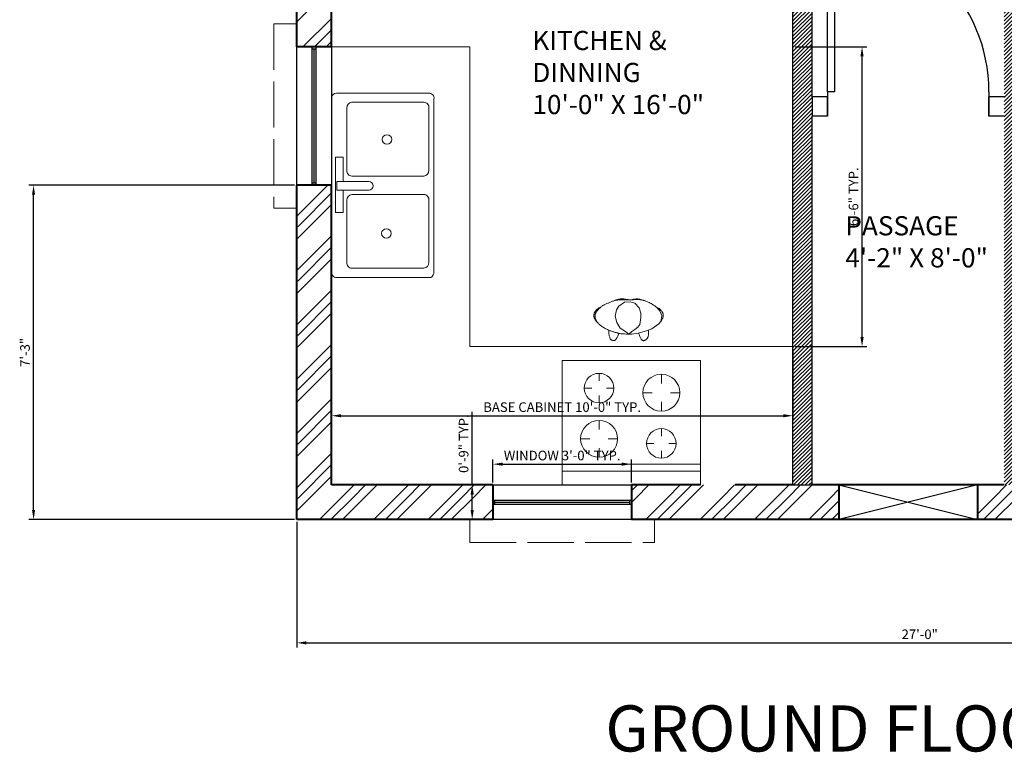
# Model space of a CAD drawing. Units: inches. Extents: x 2443635 to 2446153, y 1826255 to 1827341.
# Tile 1 of 16: x 2443635 to 2443891, y 1826801 to 1826991. Entities that reach past the tile are written whole.
import ezdxf

# ---------------------------------------------------------------- set-up
doc = ezdxf.new("R2010")
doc.units = ezdxf.units.IN
doc.linetypes.add('ACAD_ISO02W100', pattern=[15, 12, -3])
for name, color, linetype, lineweight in [('A-DIMS', 1, 'Continuous', 18), ('A-DOOR', 2, 'Continuous', 25), ('A-ENTG', 111, 'Continuous', 13), ('A-EQPM', 8, 'Continuous', 18), ('A-FLOR-CASE', 8, 'Continuous', 18), ('A-FLOR-FIXT', 9, 'Continuous', 18), ('A-ROOM', 4, 'Continuous', 18), ('A-TEXT', 4, 'Continuous', 25), ('A-WALL-EXT', 7, 'Continuous', 40), ('A-WALL-INT', 9, 'Continuous', 30), ('A-WALL-OVHD', 7, 'ACAD_ISO02W100', 18), ('A-WALL-PATT', 8, 'Continuous', 13), ('A-WINDOW', 4, 'Continuous', 25)]:
    doc.layers.add(name, color=color, linetype=linetype, lineweight=lineweight)
doc.styles.add('ATT', font='romans.shx')
doc.styles.get("Standard").update_dxf_attribs({"font": 'arial.ttf'})
doc.dimstyles.new('ISO-25', dxfattribs={"dimtxt": 2.5, "dimasz": 2.5, "dimexe": 1.25, "dimexo": 0.625, "dimtad": 1, "dimlunit": 4, "dimtxsty": 'Standard', "dimcen": 2.5, "dimadec": 0, "dimazin": 0, "dimtfac": 1, "dimtmove": 0, "dimatfit": 3, "dimfxl": 1, "dimarcsym": 0})

# ---------------------------------------------------------------- blocks, each defined once
blk = doc.blocks.new('*U2')
for p, q in [((0, 0), (0, -6)), ((40, 0), (40, -6))]:
    blk.add_line(p, q)
blk.add_lwpolyline([(0, 0), (0, 40), (1.75, 40), (1.75, 0)], close=True)
blk.add_arc((0, 0), 40, 0, 90)
blk = doc.blocks.new('11PRNG01')
at = {"color": 0, "linetype": 'ByBlock'}
for p, q in [((0, 30), (27, 30)), ((0, 0), (0, 30)), ((3, 0), (3, 30)), ((4.5, 0), (4.5, 30)), ((27, 30), (27, 0)), ((10, 26), (10, 24)), ((21, 25.2), (21, 23.6)), ((6, 22), (8, 22)), ((14, 22), (12, 22)), ((17.8, 22), (19.4, 22)), ((24.2, 22), (22.6, 22)), ((10, 18), (10, 20)), ((21, 18.8), (21, 20.4)), ((9, 11.7), (9, 10.1)), ((20, 12.5), (20, 10.5)), ((5.8, 8.5), (7.4, 8.5)), ((9, 5.3), (9, 6.9)), ((12.2, 8.5), (10.6, 8.5)), ((16, 8.5), (18, 8.5)), ((20, 4.5), (20, 6.5)), ((24, 8.5), (22, 8.5)), ((27, 0), (0, 0))]:
    blk.add_line(p, q, dxfattribs=at)
for centre, radius in [((10, 22), 4), ((21, 22), 3.2), ((9, 8.5), 3.2), ((20, 8.5), 4)]:
    blk.add_circle(centre, radius, dxfattribs=at)
at = {"color": 0, "linetype": 'ByBlock', "style": 'ATT'}
for tag, p, flags in [('ITEM', (0, -11), 3), ('ROOM_NUMBER', (0, -20), 1), ('DEPTH', (0, -29), 3), ('WIDTH', (0, -38), 3)]:
    blk.add_attdef(tag, p, '', height=6, dxfattribs=dict(at, flags=flags))
blk = doc.blocks.new('PERSON-STANDING-PLAN')
at = {"transparency": 33554687}
for p, q in [((4.62, 10.18), (4.79, 10.25)), ((4.79, 10.25), (4.96, 10.31)), ((4.96, 10.31), (5.14, 10.38)), ((5.14, 10.38), (5.33, 10.43)), ((5.33, 10.43), (5.53, 10.48)), ((5.48, 10.5), (5.36, 10.44)), ((5.69, 10.59), (5.48, 10.5)), ((5.53, 10.48), (5.74, 10.51)), ((5.91, 10.67), (5.69, 10.59)), ((5.74, 10.51), (5.95, 10.55)), ((6.13, 10.74), (5.91, 10.67)), ((5.95, 10.55), (6.17, 10.57)), ((6.35, 10.79), (6.13, 10.74)), ((6.17, 10.57), (6.39, 10.59)), ((6.57, 10.84), (6.35, 10.79)), ((6.39, 10.59), (6.61, 10.61)), ((6.79, 10.87), (6.57, 10.84)), ((6.61, 10.61), (6.83, 10.62)), ((6.99, 10.89), (6.79, 10.87)), ((6.83, 10.62), (7.05, 10.63)), ((7.18, 10.9), (6.99, 10.89)), ((7.05, 10.63), (7.26, 10.64)), ((7.38, 10.9), (7.18, 10.9)), ((7.26, 10.64), (7.47, 10.65)), ((7.57, 10.88), (7.38, 10.9)), ((7.47, 10.65), (7.68, 10.65)), ((7.78, 10.87), (7.57, 10.88)), ((7.68, 10.65), (7.87, 10.65)), ((7.99, 10.84), (7.78, 10.87)), ((7.87, 10.65), (8.06, 10.65)), ((8.22, 10.82), (7.99, 10.84)), ((8.06, 10.65), (8.23, 10.65)), ((9.71, 10.64), (8.22, 10.82)), ((8.23, 10.65), (8.39, 10.65)), ((8.39, 10.65), (8.54, 10.64)), ((8.54, 10.64), (8.67, 10.64)), ((8.67, 10.64), (8.78, 10.63)), ((8.78, 10.63), (8.89, 10.62)), ((8.89, 10.62), (8.98, 10.61)), ((8.98, 10.61), (9.08, 10.6)), ((9.08, 10.6), (9.16, 10.59)), ((9.16, 10.59), (9.25, 10.59)), ((9.25, 10.59), (9.35, 10.59)), ((9.35, 10.59), (9.44, 10.59)), ((9.44, 10.59), (9.55, 10.6)), ((9.55, 10.6), (9.66, 10.61)), ((9.9, 10.69), (9.56, 10.61)), ((9.66, 10.61), (9.78, 10.62)), ((9.78, 10.62), (9.9, 10.63)), ((10.22, 10.76), (9.9, 10.69)), ((9.9, 10.63), (10.03, 10.64)), ((10.03, 10.64), (10.16, 10.66)), ((10.16, 10.66), (10.3, 10.67)), ((10.5, 10.81), (10.22, 10.76)), ((10.3, 10.67), (10.45, 10.68)), ((10.45, 10.68), (10.61, 10.7)), ((10.76, 10.84), (10.5, 10.81)), ((10.61, 10.7), (10.76, 10.71)), ((10.99, 10.86), (10.76, 10.84)), ((10.76, 10.71), (10.92, 10.71)), ((10.92, 10.71), (11.09, 10.72)), ((11.2, 10.87), (10.99, 10.86)), ((11.09, 10.72), (11.25, 10.72)), ((11.4, 10.86), (11.2, 10.87)), ((11.25, 10.72), (11.41, 10.72)), ((11.58, 10.84), (11.4, 10.86)), ((11.41, 10.72), (11.57, 10.71)), ((11.57, 10.71), (11.73, 10.7)), ((11.76, 10.81), (11.58, 10.84)), ((11.73, 10.7), (11.89, 10.68)), ((11.93, 10.77), (11.76, 10.81)), ((11.89, 10.68), (12.04, 10.67)), ((12.11, 10.73), (11.93, 10.77)), ((12.04, 10.67), (12.19, 10.64)), ((12.29, 10.67), (12.11, 10.73)), ((12.19, 10.64), (12.34, 10.62)), ((12.48, 10.61), (12.29, 10.67)), ((12.34, 10.62), (12.48, 10.59)), ((12.68, 10.55), (12.48, 10.61)), ((12.48, 10.59), (12.62, 10.56)), ((12.62, 10.56), (12.77, 10.53)), ((12.91, 10.49), (12.68, 10.55)), ((12.77, 10.53), (12.91, 10.49)), ((12.91, 10.49), (13.05, 10.45)), ((13.17, 10.43), (12.91, 10.49)), ((13.05, 10.45), (13.2, 10.41)), ((13.2, 10.41), (13.35, 10.36)), ((13.35, 10.36), (13.51, 10.3)), ((13.51, 10.3), (13.69, 10.22)), ((0.39, 7.71), (0.32, 7.61)), ((0.48, 7.82), (0.39, 7.71)), ((0.57, 7.92), (0.48, 7.82)), ((0.67, 8.02), (0.57, 7.92)), ((0.77, 8.12), (0.67, 8.02)), ((0.76, 7.64), (0.85, 7.75)), ((0.87, 8.21), (0.77, 8.12)), ((0.85, 7.75), (0.94, 7.85)), ((0.97, 8.29), (0.87, 8.21)), ((0.94, 7.85), (1.03, 7.96)), ((1.08, 8.36), (0.97, 8.29)), ((1.03, 7.96), (1.12, 8.07)), ((1.17, 8.42), (1.08, 8.36)), ((1.12, 8.07), (1.21, 8.17)), ((1.26, 8.47), (1.17, 8.42)), ((1.21, 8.17), (1.3, 8.27)), ((1.35, 8.51), (1.26, 8.47)), ((1.3, 8.27), (1.39, 8.37)), ((1.43, 8.54), (1.35, 8.51)), ((1.39, 8.37), (1.49, 8.47)), ((1.49, 8.56), (1.43, 8.54)), ((1.55, 8.58), (1.49, 8.56)), ((1.49, 8.47), (1.59, 8.57)), ((1.59, 8.59), (1.55, 8.58)), ((1.59, 8.57), (1.69, 8.66)), ((1.62, 8.6), (1.59, 8.59)), ((1.69, 8.66), (1.79, 8.76)), ((1.79, 8.76), (1.9, 8.85)), ((1.9, 8.85), (2.01, 8.94)), ((2.01, 8.94), (2.13, 9.02)), ((2.13, 9.02), (2.26, 9.11)), ((2.26, 9.11), (2.39, 9.19)), ((2.39, 9.19), (2.54, 9.27)), ((2.54, 9.27), (2.7, 9.35)), ((2.7, 9.35), (2.86, 9.42)), ((2.86, 9.42), (3.04, 9.5)), ((3.04, 9.5), (3.21, 9.57)), ((3.21, 9.57), (3.39, 9.65)), ((3.39, 9.65), (3.58, 9.72)), ((3.58, 9.72), (3.76, 9.79)), ((3.76, 9.79), (3.94, 9.87)), ((3.94, 9.87), (4.11, 9.95)), ((4.11, 9.95), (4.28, 10.02)), ((4.28, 10.02), (4.45, 10.1)), ((4.45, 10.1), (4.62, 10.18)), ((5.88, 8.02), (5.48, 6.38)), ((6.48, 9.01), (5.88, 8.02)), ((7.91, 9.98), (6.48, 9.01)), ((9.39, 10.13), (7.91, 9.98)), ((10.63, 9.72), (9.39, 10.13)), ((11.79, 8.58), (10.63, 9.72)), ((12.18, 7.14), (11.79, 8.58)), ((13.69, 10.22), (13.89, 10.14)), ((13.89, 10.14), (14.11, 10.04)), ((14.11, 10.04), (14.35, 9.93)), ((14.35, 9.93), (14.61, 9.79)), ((14.61, 9.79), (14.89, 9.64)), ((14.89, 9.64), (15.18, 9.47)), ((15.18, 9.47), (15.49, 9.28)), ((15.49, 9.28), (15.8, 9.07)), ((15.8, 9.07), (16.12, 8.84)), ((16.12, 8.84), (16.44, 8.59)), ((16.26, 8.74), (17.17, 7.78)), ((16.44, 8.59), (16.61, 8.53)), ((16.61, 8.53), (16.77, 8.45)), ((16.77, 8.45), (16.94, 8.35)), ((16.94, 8.35), (17.1, 8.23)), ((17.1, 8.23), (17.24, 8.1)), ((17.17, 7.78), (17.68, 6.58)), ((17.24, 8.1), (17.38, 7.96)), ((17.38, 7.96), (17.51, 7.82)), ((17.51, 7.82), (17.61, 7.69)), ((17.61, 7.69), (17.7, 7.56)), ((0.01, 6.79), (0, 6.71)), ((0, 6.71), (0, 6.61)), ((0, 6.61), (0, 6.52)), ((0, 6.52), (0, 6.42)), ((0, 6.42), (0.01, 6.33)), ((0.02, 6.88), (0.01, 6.79)), ((0.01, 6.33), (0.02, 6.22)), ((0.04, 6.97), (0.02, 6.88)), ((0.02, 6.22), (0.04, 6.12)), ((0.06, 7.06), (0.04, 6.97)), ((0.04, 6.12), (0.06, 6)), ((0.08, 7.15), (0.06, 7.06)), ((0.06, 6), (0.1, 5.88)), ((0.11, 7.23), (0.08, 7.15)), ((0.1, 5.88), (0.15, 5.75)), ((0.15, 7.33), (0.11, 7.23)), ((0.2, 7.42), (0.15, 7.33)), ((0.15, 5.75), (0.23, 5.6)), ((0.25, 7.51), (0.2, 7.42)), ((0.23, 5.6), (0.33, 5.43)), ((0.32, 7.61), (0.25, 7.51)), ((0.28, 6.52), (0.29, 6.66)), ((0.29, 6.38), (0.28, 6.52)), ((0.29, 6.66), (0.31, 6.8)), ((0.3, 6.24), (0.29, 6.38)), ((0.32, 6.09), (0.3, 6.24)), ((0.31, 6.8), (0.35, 6.93)), ((0.35, 5.95), (0.32, 6.09)), ((0.33, 5.43), (0.48, 5.23)), ((0.35, 6.93), (0.4, 7.06)), ((0.39, 5.81), (0.35, 5.95)), ((0.43, 5.68), (0.39, 5.81)), ((0.4, 7.06), (0.46, 7.18)), ((0.48, 5.55), (0.43, 5.68)), ((0.46, 7.18), (0.52, 7.3)), ((0.53, 5.42), (0.48, 5.55)), ((0.48, 5.23), (0.67, 5.01)), ((0.52, 7.3), (0.6, 7.41)), ((0.58, 5.3), (0.53, 5.42)), ((0.64, 5.19), (0.58, 5.3)), ((0.6, 7.41), (0.68, 7.53)), ((0.7, 5.07), (0.64, 5.19)), ((0.68, 7.53), (0.76, 7.64)), ((5.48, 6.38), (5.95, 4.72)), ((11.9, 4.25), (12.22, 6.07)), ((12.22, 6.07), (12.18, 7.14)), ((17.68, 6.58), (17.36, 5.01)), ((17.54, 5.23), (17.36, 5)), ((17.68, 5.42), (17.54, 5.23)), ((17.78, 5.6), (17.68, 5.42)), ((17.7, 7.56), (17.78, 7.45)), ((17.78, 7.45), (17.84, 7.34)), ((17.86, 5.75), (17.78, 5.6)), ((17.84, 7.34), (17.88, 7.24)), ((17.91, 5.88), (17.86, 5.75)), ((17.88, 7.24), (17.92, 7.15)), ((17.94, 6), (17.91, 5.88)), ((17.92, 7.15), (17.95, 7.06)), ((17.96, 6.12), (17.94, 6)), ((17.95, 7.06), (17.97, 6.97)), ((17.98, 6.22), (17.96, 6.12)), ((17.97, 6.97), (17.98, 6.88)), ((17.98, 6.88), (17.99, 6.79)), ((17.99, 6.33), (17.98, 6.22)), ((17.99, 6.79), (18, 6.71)), ((18, 6.42), (17.99, 6.33)), ((18, 6.71), (18.01, 6.61)), ((18.01, 6.52), (18, 6.42)), ((18.01, 6.61), (18.01, 6.52)), ((0.67, 5.01), (0.91, 4.75)), ((0.77, 4.96), (0.7, 5.07)), ((0.85, 4.85), (0.77, 4.96)), ((0.93, 4.74), (0.85, 4.85)), ((1.01, 4.63), (0.93, 4.74)), ((1.1, 4.52), (1.01, 4.63)), ((1.21, 4.41), (1.1, 4.52)), ((1.32, 4.3), (1.21, 4.41)), ((1.44, 4.19), (1.32, 4.3)), ((1.57, 4.08), (1.44, 4.19)), ((1.72, 3.96), (1.57, 4.08)), ((1.88, 3.84), (1.72, 3.96)), ((2.06, 3.71), (1.88, 3.84)), ((2.26, 3.59), (2.06, 3.71)), ((2.46, 3.46), (2.26, 3.59)), ((2.67, 3.34), (2.46, 3.46)), ((2.89, 3.21), (2.67, 3.34)), ((3.11, 3.09), (2.89, 3.21)), ((3.33, 2.98), (3.11, 3.09)), ((3.56, 2.87), (3.33, 2.98)), ((3.77, 2.77), (3.56, 2.87)), ((3.99, 2.68), (3.77, 2.77)), ((3.86, 2.7), (3.84, 2.5)), ((4.2, 2.6), (3.99, 2.68)), ((4.4, 2.52), (4.2, 2.6)), ((5.95, 4.72), (6.81, 3.29)), ((6.81, 3.29), (8.17, 2.41)), ((9.82, 2.41), (10.66, 2.88)), ((10.66, 2.88), (11.44, 3.53)), ((11.44, 3.53), (11.9, 4.25)), ((15.08, 3.08), (13.68, 2.54)), ((14.17, 2.51), (14.14, 2.7)), ((16.88, 4.4), (15.08, 3.08)), ((17.36, 5.01), (16.88, 4.4)), ((17.36, 5), (17.14, 4.74)), ((3.84, 2.5), (3.84, 2.27)), ((3.84, 2.27), (3.86, 2.03)), ((3.86, 2.03), (3.89, 1.79)), ((3.89, 1.79), (3.93, 1.54)), ((3.93, 1.54), (3.98, 1.3)), ((3.98, 1.3), (4.03, 1.08)), ((4.03, 1.08), (4.09, 0.89)), ((4.09, 0.89), (4.14, 0.73)), ((4.14, 0.73), (4.19, 0.59)), ((4.19, 0.59), (4.24, 0.49)), ((4.24, 0.49), (4.29, 0.4)), ((4.29, 0.4), (4.34, 0.34)), ((4.34, 0.34), (4.39, 0.28)), ((4.39, 0.28), (4.45, 0.24)), ((4.6, 2.45), (4.4, 2.52)), ((4.45, 0.24), (4.51, 0.2)), ((4.51, 0.2), (4.57, 0.17)), ((4.57, 0.17), (4.64, 0.14)), ((4.8, 2.38), (4.6, 2.45)), ((4.64, 0.14), (4.72, 0.11)), ((4.72, 0.11), (4.79, 0.09)), ((4.79, 0.09), (4.86, 0.07)), ((5, 2.32), (4.8, 2.38)), ((4.86, 0.07), (4.93, 0.05)), ((4.93, 0.05), (5, 0.04)), ((5.19, 2.26), (5, 2.32)), ((5, 0.04), (5.07, 0.03)), ((5.07, 0.03), (5.13, 0.03)), ((5.13, 0.03), (5.19, 0.03)), ((5.38, 2.2), (5.19, 2.26)), ((5.19, 0.03), (5.24, 0.03)), ((5.24, 0.03), (5.29, 0.04)), ((5.29, 0.04), (5.34, 0.05)), ((5.34, 0.05), (5.39, 0.06)), ((5.56, 2.15), (5.38, 2.2)), ((5.39, 0.06), (5.43, 0.08)), ((5.43, 0.08), (5.47, 0.11)), ((5.47, 0.11), (5.51, 0.13)), ((5.51, 0.13), (5.55, 0.16)), ((5.55, 0.16), (5.59, 0.2)), ((5.74, 2.09), (5.56, 2.15)), ((5.59, 0.2), (5.63, 0.24)), ((5.63, 0.24), (5.68, 0.29)), ((5.68, 0.29), (5.72, 0.35)), ((5.72, 0.35), (5.77, 0.42)), ((5.92, 2.05), (5.74, 2.09)), ((5.77, 0.42), (5.82, 0.5)), ((5.82, 0.5), (5.88, 0.59)), ((5.88, 0.59), (5.94, 0.7)), ((6.09, 2), (5.92, 2.05)), ((5.94, 0.7), (6.01, 0.83)), ((6.01, 0.83), (6.09, 0.99)), ((6.25, 1.96), (6.09, 2)), ((6.09, 0.99), (6.17, 1.17)), ((6.17, 1.17), (6.26, 1.39)), ((6.41, 1.92), (6.25, 1.96)), ((6.26, 1.39), (6.36, 1.65)), ((6.36, 1.65), (6.46, 1.91)), ((6.55, 1.89), (6.41, 1.92)), ((6.7, 1.86), (6.55, 1.89)), ((6.85, 1.83), (6.7, 1.86)), ((7.04, 1.81), (6.85, 1.83)), ((7.27, 1.79), (7.04, 1.81)), ((7.57, 1.77), (7.27, 1.79)), ((7.97, 1.75), (7.57, 1.77)), ((8.47, 1.73), (7.97, 1.75)), ((8.17, 2.41), (9.1, 1.71)), ((9.1, 1.71), (8.47, 1.73)), ((9.1, 1.71), (9.82, 2.41)), ((9.89, 1.71), (9.1, 1.71)), ((11.53, 1.95), (9.89, 1.71)), ((13.68, 2.54), (11.53, 1.95)), ((11.63, 1.91), (11.74, 1.61)), ((11.74, 1.61), (11.85, 1.34)), ((11.85, 1.34), (11.95, 1.1)), ((11.95, 1.1), (12.05, 0.89)), ((12.05, 0.89), (12.13, 0.71)), ((12.13, 0.71), (12.22, 0.55)), ((12.22, 0.55), (12.29, 0.41)), ((12.29, 0.41), (12.37, 0.3)), ((12.37, 0.3), (12.44, 0.21)), ((12.44, 0.21), (12.51, 0.14)), ((12.51, 0.14), (12.58, 0.08)), ((12.58, 0.08), (12.64, 0.04)), ((12.64, 0.04), (12.71, 0.02)), ((12.71, 0.02), (12.77, 0.01)), ((12.77, 0.01), (12.84, 0)), ((12.84, 0), (12.9, 0)), ((12.9, 0), (12.97, 0.01)), ((12.97, 0.01), (13.03, 0.02)), ((13.03, 0.02), (13.1, 0.04)), ((13.1, 0.04), (13.17, 0.06)), ((13.17, 0.06), (13.24, 0.09)), ((13.24, 0.09), (13.3, 0.12)), ((13.3, 0.12), (13.37, 0.15)), ((13.37, 0.15), (13.43, 0.18)), ((13.43, 0.18), (13.49, 0.22)), ((13.49, 0.22), (13.55, 0.26)), ((13.55, 0.26), (13.61, 0.31)), ((13.61, 0.31), (13.67, 0.35)), ((13.67, 0.35), (13.72, 0.41)), ((13.72, 0.41), (13.77, 0.47)), ((13.77, 0.47), (13.82, 0.53)), ((13.82, 0.53), (13.87, 0.6)), ((13.87, 0.6), (13.92, 0.67)), ((13.92, 0.67), (13.96, 0.75)), ((13.96, 0.75), (14.01, 0.84)), ((14.01, 0.84), (14.05, 0.94)), ((14.05, 0.94), (14.08, 1.04)), ((14.08, 1.04), (14.11, 1.15)), ((14.11, 1.15), (14.14, 1.27)), ((14.14, 1.27), (14.17, 1.4)), ((14.19, 2.34), (14.17, 2.51)), ((14.17, 1.4), (14.19, 1.54)), ((14.2, 2.16), (14.19, 2.34)), ((14.19, 1.54), (14.2, 1.68)), ((14.21, 2), (14.2, 2.16)), ((14.2, 1.68), (14.21, 1.83)), ((14.21, 1.83), (14.21, 2))]:
    blk.add_line(p, q, dxfattribs=at)
blk = doc.blocks.new('BASE-CABINET-L-PLAN')
at = {"transparency": 33554687}
for p, q in [((0, 78), (36, 78)), ((36, 0), (36, 78)), ((120, 0), (36, 0))]:
    blk.add_line(p, q, dxfattribs=at)
blk = doc.blocks.new('WIN-36-PLAN')
at = {"transparency": 33554687}
for p, q in [((0, 9), (36, 9)), ((0, 0), (0, 9)), ((36, 9), (36, 0)), ((0, 5), (36, 5)), ((0, 4), (36, 4)), ((0.5, 4), (0.5, 5)), ((0.5, 4.5), (35.5, 4.5)), ((35.5, 5), (35.5, 4)), ((36, 0), (0, 0))]:
    blk.add_line(p, q, dxfattribs=at)
blk = doc.blocks.new('WINDOW-HOOD-48-PLAN')
at = {"transparency": 33554687}
for p, q in [((0, 6), (0, 0)), ((48, 0), (48, 6)), ((0, 0), (48, 0))]:
    blk.add_line(p, q, dxfattribs=at)
blk = doc.blocks.new('*D56')
at = {"layer": 'A-DIMS', "color": 0, "lineweight": -2, "transparency": 16777216}
for p, q in [((2443758.09, 1826870.91), (2443758.09, 1826876.94)), ((2443760.59, 1826875.69), (2443791.59, 1826875.69)), ((2443794.09, 1826870.91), (2443794.09, 1826876.94))]:
    blk.add_line(p, q, dxfattribs=at)
at = {"layer": 'A-DIMS', "color": 0, "transparency": 16777216}
for points in [[(2443760.59, 1826876.1), (2443760.59, 1826875.27), (2443758.09, 1826875.69)], [(2443791.59, 1826876.1), (2443791.59, 1826875.27), (2443794.09, 1826875.69)]]:
    blk.add_solid(points, dxfattribs=at)
at = {"layer": 'Defpoints', "color": 0, "transparency": 16777216}
for p in [(2443794.09, 1826875.69), (2443758.09, 1826870.29), (2443794.09, 1826870.29)]:
    blk.add_point(p, dxfattribs=at)
at = {"layer": 'A-DIMS', "color": 0, "transparency": 16777216, "insert": (2443776.09, 1826877.61), "char_height": 2.5, "attachment_point": 5}
blk.add_mtext('WINDOW 3\'-0" TYP.', dxfattribs=at)
blk = doc.blocks.new('*D57')
at = {"layer": 'A-DIMS', "color": 0, "lineweight": -2, "transparency": 16777216}
for p, q in [((2443752.69, 1826870.29), (2443752.69, 1826889.28)), ((2443757.46, 1826870.29), (2443751.44, 1826870.29)), ((2443752.69, 1826863.79), (2443752.69, 1826867.79)), ((2443757.46, 1826861.29), (2443751.44, 1826861.29))]:
    blk.add_line(p, q, dxfattribs=at)
at = {"layer": 'A-DIMS', "color": 0, "transparency": 16777216}
for points in [[(2443752.27, 1826867.79), (2443753.11, 1826867.79), (2443752.69, 1826870.29)], [(2443752.27, 1826863.79), (2443753.11, 1826863.79), (2443752.69, 1826861.29)]]:
    blk.add_solid(points, dxfattribs=at)
at = {"layer": 'Defpoints', "color": 0, "transparency": 16777216}
for p in [(2443752.69, 1826870.29), (2443758.09, 1826870.29), (2443758.09, 1826861.29)]:
    blk.add_point(p, dxfattribs=at)
at = {"layer": 'A-DIMS', "color": 0, "transparency": 16777216, "insert": (2443750.79, 1826881.03), "char_height": 2.5, "attachment_point": 5, "rotation": 90}
blk.add_mtext('0\'-9" TYP.', dxfattribs=at)
blk = doc.blocks.new('*D76')
at = {"layer": 'A-DIMS', "color": 0, "lineweight": -2, "transparency": 16777216}
for p, q in [((2443716.09, 1826905.66), (2443716.09, 1826887.04)), ((2443836.09, 1826905.66), (2443836.09, 1826887.04)), ((2443718.59, 1826888.29), (2443833.59, 1826888.29))]:
    blk.add_line(p, q, dxfattribs=at)
at = {"layer": 'A-DIMS', "color": 0, "transparency": 16777216}
for points in [[(2443718.59, 1826888.7), (2443718.59, 1826887.87), (2443716.09, 1826888.29)], [(2443833.59, 1826888.7), (2443833.59, 1826887.87), (2443836.09, 1826888.29)]]:
    blk.add_solid(points, dxfattribs=at)
at = {"layer": 'Defpoints', "color": 0, "transparency": 16777216}
for p in [(2443716.09, 1826906.29), (2443836.09, 1826906.29), (2443836.09, 1826888.29)]:
    blk.add_point(p, dxfattribs=at)
at = {"layer": 'A-DIMS', "color": 0, "transparency": 16777216, "insert": (2443776.09, 1826890.21), "char_height": 2.5, "attachment_point": 5}
blk.add_mtext('BASE CABINET 10\'-0" TYP.', dxfattribs=at)
blk = doc.blocks.new('*D77')
at = {"layer": 'A-DIMS', "color": 0, "lineweight": -2, "transparency": 16777216}
for p, q in [((2443836.71, 1826984.29), (2443855.34, 1826984.29)), ((2443854.09, 1826908.79), (2443854.09, 1826981.79)), ((2443836.71, 1826906.29), (2443855.34, 1826906.29))]:
    blk.add_line(p, q, dxfattribs=at)
at = {"layer": 'A-DIMS', "color": 0, "transparency": 16777216}
for points in [[(2443853.67, 1826981.79), (2443854.51, 1826981.79), (2443854.09, 1826984.29)], [(2443853.67, 1826908.79), (2443854.51, 1826908.79), (2443854.09, 1826906.29)]]:
    blk.add_solid(points, dxfattribs=at)
at = {"layer": 'Defpoints', "color": 0, "transparency": 16777216}
for p in [(2443836.09, 1826984.29), (2443854.09, 1826984.29), (2443836.09, 1826906.29)]:
    blk.add_point(p, dxfattribs=at)
at = {"layer": 'A-DIMS', "color": 0, "transparency": 16777216, "insert": (2443852.19, 1826945.29), "char_height": 2.5, "attachment_point": 5, "rotation": 90}
blk.add_mtext('6\'-6" TYP.', dxfattribs=at)
blk = doc.blocks.new('*D90')
at = {"layer": 'A-DIMS', "color": 0, "lineweight": -2, "transparency": 16777216}
for p, q in [((2443707.09, 1826860.66), (2443707.09, 1826827.94)), ((2444031.09, 1826860.66), (2444031.09, 1826827.94)), ((2443709.59, 1826829.19), (2444028.59, 1826829.19))]:
    blk.add_line(p, q, dxfattribs=at)
at = {"layer": 'A-DIMS', "color": 0, "transparency": 16777216}
for points in [[(2443709.59, 1826829.6), (2443709.59, 1826828.77), (2443707.09, 1826829.19)], [(2444028.59, 1826829.6), (2444028.59, 1826828.77), (2444031.09, 1826829.19)]]:
    blk.add_solid(points, dxfattribs=at)
at = {"layer": 'Defpoints', "color": 0, "transparency": 16777216}
for p in [(2443707.09, 1826861.29), (2444031.09, 1826861.29), (2444031.09, 1826829.19)]:
    blk.add_point(p, dxfattribs=at)
at = {"layer": 'A-DIMS', "color": 0, "transparency": 16777216, "insert": (2443869.09, 1826831.09), "char_height": 2.5, "attachment_point": 5}
blk.add_mtext('27\'-0"', dxfattribs=at)
blk = doc.blocks.new('*D93')
at = {"layer": 'A-DIMS', "color": 0, "lineweight": -2, "transparency": 16777216}
for p, q in [((2443706.46, 1826948.29), (2443637.36, 1826948.29)), ((2443638.61, 1826863.79), (2443638.61, 1826945.79)), ((2443706.46, 1826861.29), (2443637.36, 1826861.29))]:
    blk.add_line(p, q, dxfattribs=at)
at = {"layer": 'A-DIMS', "color": 0, "transparency": 16777216}
for points in [[(2443638.19, 1826945.79), (2443639.02, 1826945.79), (2443638.61, 1826948.29)], [(2443638.19, 1826863.79), (2443639.02, 1826863.79), (2443638.61, 1826861.29)]]:
    blk.add_solid(points, dxfattribs=at)
at = {"layer": 'Defpoints', "color": 0, "transparency": 16777216}
for p in [(2443638.61, 1826948.29), (2443707.09, 1826948.29), (2443707.09, 1826861.29)]:
    blk.add_point(p, dxfattribs=at)
at = {"layer": 'A-DIMS', "color": 0, "transparency": 16777216, "insert": (2443636.7, 1826904.79), "char_height": 2.5, "attachment_point": 5, "rotation": 90}
blk.add_mtext('7\'-3"', dxfattribs=at)

msp = doc.modelspace()

# ---------------------------------------------------------------- hatches: boundary and pattern name
at = {"layer": 'A-WALL-PATT'}
h = msp.add_hatch(dxfattribs=at)
h.set_pattern_fill('GOST_GROUND', color=256)
h.paths.add_polyline_path([(2443848.09, 1826870.288), (2443841.09, 1826870.288), (2443836.09, 1826870.288), (2443794.09, 1826870.288), (2443794.09, 1826861.288), (2443848.09, 1826861.288)])
h.paths.add_polyline_path([(2443935.09, 1826870.288), (2443896.09, 1826870.288), (2443891.09, 1826870.288), (2443884.09, 1826870.288), (2443884.09, 1826861.288), (2443935.09, 1826861.288)])
h.paths.add_polyline_path([(2444031.09, 1826999.288), (2444022.09, 1826999.288), (2444022.09, 1826995.288), (2444022.09, 1826990.288), (2444022.09, 1826870.288), (2443983.09, 1826870.288), (2443983.09, 1826861.288), (2444031.09, 1826861.288)])
h.paths.add_polyline_path([(2443758.09, 1826870.288), (2443716.09, 1826870.288), (2443716.09, 1826925.457, -0.0618154), (2443716.09, 1826925.788), (2443716.09, 1826948.288), (2443707.09, 1826948.288), (2443707.09, 1826861.288), (2443758.09, 1826861.288)])
h.paths.add_polyline_path([(2443716.09, 1827062.288), (2443716.09, 1827067.288), (2443716.09, 1827147.288), (2443716.09, 1827152.288), (2443716.09, 1827194.288), (2443707.09, 1827194.288), (2443707.09, 1826984.288), (2443716.09, 1826984.288)])
h.paths.add_polyline_path([(2443716.09, 1827296.288), (2443836.09, 1827296.288), (2443841.09, 1827296.288), (2443860.09, 1827296.288), (2443860.09, 1827305.288), (2443707.09, 1827305.288), (2443707.09, 1827254.288), (2443716.09, 1827254.288)])
h.paths.add_polyline_path([(2444031.09, 1827305.288), (2443878.09, 1827305.288), (2443878.09, 1827296.288), (2443881.588, 1827296.288), (2443897.09, 1827296.288), (2443902.09, 1827296.288), (2444022.09, 1827296.288), (2444022.09, 1827284.209), (2444022.09, 1827254.288), (2444031.09, 1827254.288)])
h.paths.add_polyline_path([(2444031.09, 1827194.288), (2444022.09, 1827194.288), (2444022.09, 1827152.288), (2444022.09, 1827147.288), (2444022.09, 1827113.953), (2444022.096, 1827113.948), (2444022.084, 1827080.628), (2444022.09, 1827047.288), (2444031.09, 1827047.288)])
h = msp.add_hatch(dxfattribs=at)
h.set_pattern_fill('JIS_WOOD', color=256)
h.paths.add_polyline_path([(2443841.09, 1827296.288), (2443836.09, 1827296.288), (2443836.09, 1827192.288), (2443841.09, 1827192.288), (2443841.09, 1827195.288), (2443861.09, 1827195.288), (2443861.09, 1827200.288), (2443841.09, 1827200.288)])
h.paths.add_polyline_path([(2443902.09, 1827296.288), (2443897.09, 1827296.288), (2443897.09, 1827200.288), (2443891.09, 1827200.288), (2443891.09, 1827195.288), (2443897.09, 1827195.288), (2443897.09, 1827192.288), (2443902.09, 1827192.288)])
h.paths.add_polyline_path([(2444022.09, 1827147.288), (2444022.09, 1827152.288), (2443902.09, 1827152.288), (2443902.09, 1827156.288), (2443897.09, 1827156.288), (2443897.09, 1827147.288)])
h.paths.add_polyline_path([(2443716.09, 1827152.288), (2443716.09, 1827147.288), (2443841.09, 1827147.288), (2443841.09, 1827156.288), (2443836.09, 1827156.288), (2443836.09, 1827152.288)])
h.paths.add_polyline_path([(2443836.09, 1827062.288), (2443836.09, 1827056.288), (2443841.09, 1827056.288), (2443841.09, 1827067.288), (2443716.09, 1827067.288), (2443716.09, 1827062.288)])
h.paths.add_polyline_path([(2443841.09, 1827020.288), (2443836.09, 1827020.288), (2443836.09, 1826870.288), (2443841.09, 1826870.288), (2443841.09, 1826966.288), (2443841.09, 1826971.288)])
h.paths.add_polyline_path([(2443896.09, 1826990.288), (2443980.09, 1826990.288), (2443980.09, 1826995.288), (2443891.09, 1826995.288), (2443891.09, 1826971.288), (2443891.09, 1826966.288), (2443891.09, 1826870.288), (2443896.09, 1826870.288)])

# ---------------------------------------------------------------- linework, layer by layer
at = {"layer": 'A-DOOR'}
for p, q in [((2443848.09, 1826870.288), (2443884.09, 1826861.288)), ((2443884.09, 1826870.288), (2443848.09, 1826861.288)), ((2443848.09, 1826861.288), (2443848.09, 1826870.288)), ((2443884.09, 1826861.288), (2443884.09, 1826870.288))]:
    msp.add_line(p, q, dxfattribs=at)
at = {"layer": 'A-FLOR-FIXT'}
for p, q in [((2443716.09, 1826925.788), (2443716.09, 1826970.788)), ((2443717.423, 1826972.279), (2443741.423, 1826972.279)), ((2443721.423, 1826969.879), (2443740.09, 1826969.879)), ((2443742.757, 1826970.779), (2443742.757, 1826925.788)), ((2443720.09, 1826952.179), (2443720.09, 1826968.379)), ((2443741.423, 1826968.379), (2443741.423, 1826952.179)), ((2443717.174, 1826955.55), (2443717.174, 1826941.15)), ((2443719.173, 1826955.55), (2443717.174, 1826955.55)), ((2443719.173, 1826949.262), (2443719.173, 1826955.55)), ((2443725.79, 1826949.262), (2443717.519, 1826949.262)), ((2443717.519, 1826949.262), (2443717.519, 1826947.027)), ((2443740.09, 1826950.679), (2443721.423, 1826950.679)), ((2443717.519, 1826947.027), (2443725.79, 1826947.027)), ((2443719.173, 1826941.15), (2443719.173, 1826947.027)), ((2443720.09, 1826928.179), (2443720.09, 1826944.379)), ((2443721.423, 1826945.879), (2443740.09, 1826945.879)), ((2443741.423, 1826944.379), (2443741.423, 1826928.179)), ((2443717.174, 1826941.15), (2443719.173, 1826941.15)), ((2443740.09, 1826926.679), (2443721.423, 1826926.679)), ((2443741.923, 1826924.288), (2443717.423, 1826924.279))]:
    msp.add_line(p, q, dxfattribs=at)
for centre in [(2443730.534, 1826960.197), (2443730.366, 1826935.745)]:
    msp.add_circle(centre, 1.233, dxfattribs=at)
for centre, radius, start, end in [((2443717.591, 1826970.788), 1.501, 96.40919, 180.00001), ((2443721.6, 1826968.379), 1.51, 96.73295, 179.99997), ((2443740.09, 1826968.537), 1.343, 353.26708, 89.99999), ((2443741.423, 1826970.937), 1.343, 353.26708, 89.99999), ((2443721.423, 1826952.022), 1.343, 173.26708, 269.99999), ((2443739.913, 1826952.179), 1.51, 276.73295, 359.99997), ((2443725.79, 1826948.145), 1.117, 270, 90), ((2443721.6, 1826944.379), 1.51, 96.73295, 179.99997), ((2443740.09, 1826944.537), 1.343, 353.26708, 89.99999), ((2443721.423, 1826928.022), 1.343, 173.26708, 269.99999), ((2443739.913, 1826928.179), 1.51, 276.73295, 359.99997), ((2443717.423, 1826925.623), 1.343, 172.92547, 270.01993), ((2443740.99, 1826925.788), 1.767, 301.89079, 360)]:
    msp.add_arc(centre, radius, start, end, dxfattribs=at)
at = {"layer": 'A-WALL-EXT'}
for p, q in [((2443707.09, 1826984.288), (2443707.09, 1827194.288)), ((2443716.09, 1826984.288), (2443716.09, 1827062.288)), ((2443716.09, 1826984.288), (2443707.09, 1826984.288)), ((2443707.09, 1826861.288), (2443707.09, 1826948.288)), ((2443716.09, 1826948.288), (2443707.09, 1826948.288)), ((2443716.09, 1826870.288), (2443716.09, 1826948.288)), ((2443758.09, 1826870.288), (2443716.09, 1826870.288)), ((2443758.09, 1826870.288), (2443758.09, 1826861.288)), ((2443794.09, 1826870.288), (2443794.09, 1826861.288)), ((2443812.09, 1826870.288), (2443794.09, 1826870.288)), ((2443836.09, 1826870.288), (2443821.09, 1826870.288)), ((2443891.09, 1826870.288), (2443841.09, 1826870.288)), ((2443848.09, 1826870.288), (2443848.09, 1826861.288)), ((2443884.09, 1826870.288), (2443884.09, 1826861.288)), ((2443758.09, 1826861.288), (2443707.09, 1826861.288)), ((2443935.09, 1826861.288), (2443794.09, 1826861.288))]:
    msp.add_line(p, q, dxfattribs=at)
at = {"layer": 'A-WALL-INT'}
for p, q in [((2443836.09, 1826870.288), (2443836.09, 1827020.288)), ((2443841.09, 1826971.288), (2443841.09, 1827020.288)), ((2443841.09, 1826971.288), (2443841.09, 1826966.288)), ((2443845.09, 1826971.288), (2443841.09, 1826971.288)), ((2443845.09, 1826966.288), (2443845.09, 1826971.288)), ((2443891.09, 1826971.288), (2443887.09, 1826971.288)), ((2443887.09, 1826966.288), (2443887.09, 1826971.288)), ((2443841.09, 1826870.288), (2443841.09, 1826966.288)), ((2443845.09, 1826966.288), (2443841.09, 1826966.288)), ((2443891.09, 1826966.288), (2443887.09, 1826966.288)), ((2443836.09, 1826870.288), (2443841.09, 1826870.288))]:
    msp.add_line(p, q, dxfattribs=at)

# ---------------------------------------------------------------- block references
at = {"layer": 'A-DOOR', "xscale": 1.05, "yscale": 1.05, "zscale": 1.05}
msp.add_blockref('*U2', (2443845.09, 1826972.588), dxfattribs=at)
at = {"layer": 'A-ENTG', "transparency": 33554687}
msp.add_blockref('PERSON-STANDING-PLAN', (2443784.359, 1826907.83), dxfattribs=at)
at = {"layer": 'A-EQPM', "xscale": 1.199999999999791, "yscale": 1.199999999999791, "zscale": 1.199999999999791, "rotation": 89.99999999999999}
msp.add_blockref('11PRNG01', (2443812.09, 1826870.288), dxfattribs=at)
at = {"layer": 'A-FLOR-CASE', "transparency": 33554687}
msp.add_blockref('BASE-CABINET-L-PLAN', (2443716.09, 1826906.288), dxfattribs=at)
at = {"layer": 'A-WALL-OVHD', "transparency": 33554687, "rotation": 270.0000000021633}
msp.add_blockref('WINDOW-HOOD-48-PLAN', (2443701.09, 1826990.288), dxfattribs=at)
at = {"layer": 'A-WALL-OVHD', "transparency": 33554687}
msp.add_blockref('WINDOW-HOOD-48-PLAN', (2443752.09, 1826855.288), dxfattribs=at)
at = {"layer": 'A-WINDOW', "transparency": 33554687, "rotation": 90.0000000020926}
msp.add_blockref('WIN-36-PLAN', (2443716.09, 1826948.288), dxfattribs=at)
at = {"layer": 'A-WINDOW', "transparency": 33554687}
msp.add_blockref('WIN-36-PLAN', (2443758.09, 1826861.288), dxfattribs=at)

# ---------------------------------------------------------------- texts
at = {"layer": 'A-ROOM', "char_height": 5, "attachment_point": 1}
for s, insert in [('KITCHEN &\\PDINNING\\P10\'-0" X 16\'-0"', (2443768.338, 1826988.457)), ('PASSAGE\\P4\'-2" X 8\'-0"', (2443849.739, 1826940.231))]:
    msp.add_mtext_dynamic_manual_height_columns(s, width=52.37406, gutter_width=12.5, heights=[0], dxfattribs=dict(at, insert=insert))
at = {"layer": 'A-TEXT', "insert": (2443787.328, 1826812.907), "char_height": 12, "attachment_point": 1}
msp.add_mtext_dynamic_manual_height_columns('GROUND FLOOR PLAN', width=201.69861, gutter_width=12.5, heights=[0], dxfattribs=at)

# ---------------------------------------------------------------- dimensions: what is measured, and where the dimension line sits
at = {"layer": 'A-DIMS', "transparency": 33554687}
for base, p1, p2, picture, middle in [((2443854.09, 1826984.288), (2443836.09, 1826906.288), (2443836.09, 1826984.288), '*D77', (2443852.188, 1826945.288)), ((2443752.69, 1826870.288), (2443758.09, 1826861.288), (2443758.09, 1826870.288), '*D57', (2443750.788, 1826881.032))]:
    dim = msp.add_linear_dim(base=base, p1=p1, p2=p2, angle=90, text='<> TYP.', dimstyle='ISO-25', override={"dimdec": 1, "dimlfac": 1, "dimrnd": 0, "dimzin": 1, "dimdsep": 46, "dimlunit": 4, "dimfrac": 2}, dxfattribs=at)
    dim.commit()
    dim.dimension.update_dxf_attribs({"geometry": picture, "text_midpoint": middle})
dim = msp.add_linear_dim(base=(2443638.607, 1826948.288), p1=(2443707.09, 1826861.288), p2=(2443707.09, 1826948.288), angle=90, dimstyle='ISO-25', override={"dimdec": 1, "dimlfac": 1, "dimrnd": 0, "dimzin": 1, "dimdsep": 46, "dimlunit": 4, "dimfrac": 2}, dxfattribs=at)
dim.commit()
dim.dimension.update_dxf_attribs({"geometry": '*D93', "text_midpoint": (2443636.704, 1826904.788)})
for base, p1, p2, text, picture, middle in [((2443836.09, 1826888.288), (2443716.09, 1826906.288), (2443836.09, 1826906.288), 'BASE CABINET <> TYP.', '*D76', (2443776.09, 1826890.206)), ((2443794.09, 1826875.688), (2443758.09, 1826870.288), (2443794.09, 1826870.288), 'WINDOW <> TYP.', '*D56', (2443776.09, 1826877.607))]:
    dim = msp.add_linear_dim(base=base, p1=p1, p2=p2, text=text, dimstyle='ISO-25', override={"dimdec": 1, "dimlfac": 1, "dimrnd": 0, "dimzin": 1, "dimdsep": 46, "dimlunit": 4, "dimfrac": 2}, dxfattribs=at)
    dim.commit()
    dim.dimension.update_dxf_attribs({"geometry": picture, "text_midpoint": middle})
dim = msp.add_linear_dim(base=(2444031.09, 1826829.188), p1=(2443707.09, 1826861.288), p2=(2444031.09, 1826861.288), dimstyle='ISO-25', override={"dimdec": 1, "dimlfac": 1, "dimrnd": 0, "dimzin": 1, "dimdsep": 46, "dimlunit": 4, "dimfrac": 2}, dxfattribs=at)
dim.commit()
dim.dimension.update_dxf_attribs({"geometry": '*D90', "text_midpoint": (2443869.09, 1826831.089)})

doc.saveas('drawing.dxf')
